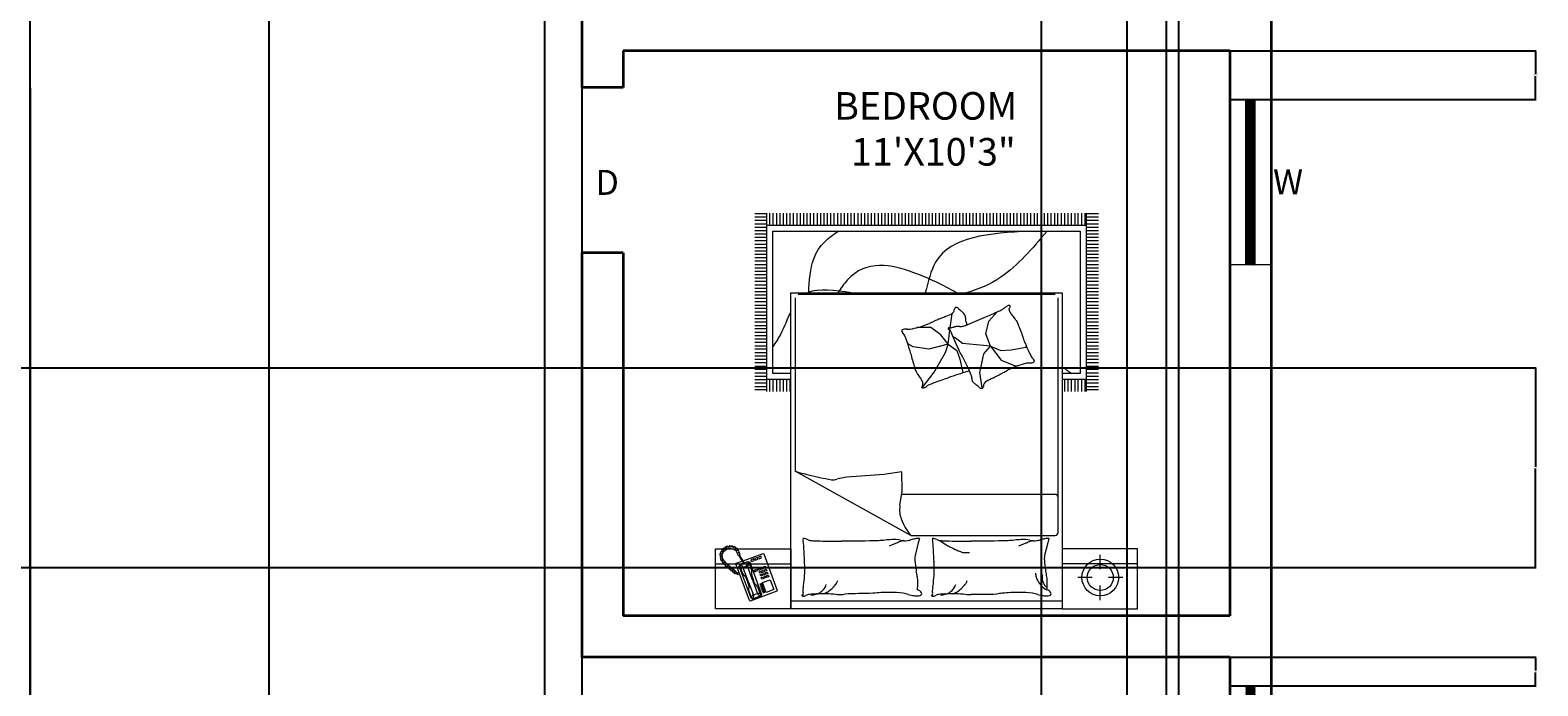
# Model space of a CAD drawing. Units: inches. Extents: x 318 to 927, y -1130 to 13.
# Tile 12 of 17: x 599 to 927, y -440 to -297. Entities that reach past the tile are written whole.
import ezdxf

# ---------------------------------------------------------------- set-up
doc = ezdxf.new("R2010")
doc.units = ezdxf.units.IN
doc.header["$MEASUREMENT"] = 0
for name, color, linetype, lineweight in [('A-ANNO-DIMS', 1, 'Continuous', 18), ('A-ANNO-IDEN', 1, 'Continuous', 13), ('A-AREA-IDEN', 8, 'Continuous', 18), ('A-GLAZ-PATT', 5, 'Continuous', 9), ('wall', 1, 'Continuous', 35), ('win', 5, 'Continuous', 18)]:
    doc.layers.add(name, color=color, linetype=linetype, lineweight=lineweight)
doc.layers.add('furniture', color=50, linetype='Continuous', lineweight=13, transparency=0.8)
doc.styles.add('DIM_FONT', font='SIMPLEX.shx', dxfattribs={"width": 0.8})
doc.styles.get("Standard").update_dxf_attribs({"font": 'arial.ttf'})
doc.dimstyles.get("Standard").update_dxf_attribs({"dimtxt": 0.18, "dimasz": 0.18, "dimexe": 0.18, "dimexo": 0.0625, "dimgap": 0.09, "dimtad": 0, "dimtih": 1, "dimtoh": 1, "dimdec": 1, "dimzin": 0, "dimdsep": 46, "dimlunit": 4, "dimtxsty": 'Standard', "dimcen": 0.09, "dimadec": 0, "dimazin": 0, "dimtfac": 1, "dimtdec": 1, "dimtofl": 0, "dimtmove": 0, "dimatfit": 3, "dimfxl": 1, "dimtolj": 1, "dimtzin": 0, "dimarcsym": 0})

# ---------------------------------------------------------------- blocks, each defined once
blk = doc.blocks.new('A$C4F634EDD')
for p, q in [((0, 2.629), (0, 2.229)), ((0.5, 2.629), (0, 2.629)), ((0.5, 2.629), (2.3, 2.629)), ((0.5, 0.529), (0.5, 2.629)), ((0.5, 2.229), (0.5, 2.629)), ((2.3, 2.629), (2.3, 0.529)), ((2.3, 2.629), (2.8, 2.629)), ((2.3, 2.229), (2.3, 2.629)), ((2.8, 2.629), (2.8, 2.229)), ((0.246, 2.57), (0.246, 2.473)), ((0.5, 2.577), (2.3, 2.577)), ((2.39, 2.507), (2.392, 2.511)), ((2.48, 2.262), (2.39, 2.507)), ((2.392, 2.511), (2.569, 2.577)), ((2.412, 2.501), (2.463, 2.52)), ((2.463, 2.52), (2.487, 2.454)), ((2.484, 2.523), (2.47, 2.518)), ((2.47, 2.518), (2.472, 2.513)), ((2.472, 2.513), (2.486, 2.518)), ((2.488, 2.513), (2.474, 2.507)), ((2.474, 2.507), (2.476, 2.502)), ((2.476, 2.502), (2.49, 2.507)), ((2.492, 2.502), (2.478, 2.497)), ((2.486, 2.518), (2.484, 2.523)), ((2.49, 2.507), (2.488, 2.513)), ((2.494, 2.497), (2.492, 2.502)), ((2.495, 2.533), (2.498, 2.545)), ((2.573, 2.319), (2.495, 2.533)), ((2.498, 2.545), (2.552, 2.564)), ((2.506, 2.545), (2.5, 2.539)), ((2.5, 2.539), (2.501, 2.531)), ((2.501, 2.531), (2.519, 2.484)), ((2.501, 2.531), (2.523, 2.521)), ((2.506, 2.545), (2.549, 2.561)), ((2.524, 2.526), (2.506, 2.545)), ((2.523, 2.521), (2.524, 2.526)), ((2.552, 2.442), (2.523, 2.521)), ((2.548, 2.535), (2.524, 2.526)), ((2.548, 2.535), (2.549, 2.561)), ((2.551, 2.532), (2.548, 2.535)), ((2.549, 2.561), (2.557, 2.56)), ((2.562, 2.554), (2.551, 2.532)), ((2.581, 2.452), (2.551, 2.532)), ((2.552, 2.564), (2.564, 2.558)), ((2.557, 2.56), (2.562, 2.554)), ((2.562, 2.554), (2.579, 2.506)), ((2.564, 2.558), (2.642, 2.346)), ((2.569, 2.577), (2.574, 2.574)), ((2.574, 2.574), (2.664, 2.33)), ((2.579, 2.506), (2.579, 2.496)), ((0.096, 2.42), (0.192, 2.42)), ((0.299, 2.42), (0.396, 2.42)), ((2.436, 2.435), (2.412, 2.501)), ((2.487, 2.454), (2.436, 2.435)), ((2.446, 2.415), (2.456, 2.418)), ((2.45, 2.404), (2.446, 2.415)), ((2.46, 2.408), (2.45, 2.404)), ((2.456, 2.418), (2.46, 2.408)), ((2.463, 2.421), (2.474, 2.425)), ((2.467, 2.41), (2.463, 2.421)), ((2.478, 2.414), (2.467, 2.41)), ((2.471, 2.402), (2.481, 2.405)), ((2.474, 2.425), (2.478, 2.414)), ((2.478, 2.497), (2.48, 2.491)), ((2.48, 2.491), (2.494, 2.497)), ((2.481, 2.428), (2.492, 2.431)), ((2.485, 2.417), (2.481, 2.428)), ((2.481, 2.405), (2.485, 2.395)), ((2.496, 2.491), (2.482, 2.486)), ((2.482, 2.486), (2.484, 2.481)), ((2.484, 2.481), (2.498, 2.486)), ((2.496, 2.421), (2.485, 2.417)), ((2.5, 2.481), (2.486, 2.475)), ((2.486, 2.475), (2.488, 2.47)), ((2.488, 2.47), (2.502, 2.475)), ((2.488, 2.408), (2.499, 2.412)), ((2.492, 2.397), (2.488, 2.408)), ((2.504, 2.47), (2.49, 2.465)), ((2.49, 2.465), (2.491, 2.46)), ((2.491, 2.46), (2.506, 2.465)), ((2.492, 2.431), (2.496, 2.421)), ((2.498, 2.486), (2.496, 2.491)), ((2.499, 2.412), (2.503, 2.401)), ((2.502, 2.475), (2.5, 2.481)), ((2.506, 2.465), (2.504, 2.47)), ((2.519, 2.484), (2.526, 2.476)), ((2.526, 2.476), (2.534, 2.469)), ((2.534, 2.469), (2.541, 2.457)), ((2.541, 2.457), (2.547, 2.44)), ((2.559, 2.406), (2.547, 2.44)), ((2.552, 2.442), (2.587, 2.346)), ((2.562, 2.393), (2.559, 2.406)), ((2.579, 2.496), (2.577, 2.485)), ((2.577, 2.485), (2.579, 2.472)), ((2.579, 2.472), (2.586, 2.454)), ((2.581, 2.452), (2.616, 2.356)), ((2.598, 2.42), (2.586, 2.454)), ((2.605, 2.409), (2.598, 2.42)), ((2.613, 2.402), (2.605, 2.409)), ((2.62, 2.394), (2.613, 2.402)), ((0, 2.33), (0.5, 2.33)), ((0.246, 2.366), (0.246, 2.27)), ((2.8, 2.33), (2.3, 2.33)), ((2.453, 2.395), (2.463, 2.399)), ((2.457, 2.384), (2.453, 2.395)), ((2.467, 2.388), (2.457, 2.384)), ((2.46, 2.376), (2.471, 2.379)), ((2.464, 2.365), (2.46, 2.376)), ((2.463, 2.399), (2.467, 2.388)), ((2.475, 2.369), (2.464, 2.365)), ((2.467, 2.356), (2.478, 2.36)), ((2.471, 2.345), (2.467, 2.356)), ((2.474, 2.391), (2.471, 2.402)), ((2.471, 2.379), (2.475, 2.369)), ((2.482, 2.349), (2.471, 2.345)), ((2.485, 2.395), (2.474, 2.391)), ((2.478, 2.382), (2.488, 2.386)), ((2.482, 2.371), (2.478, 2.382)), ((2.478, 2.36), (2.482, 2.349)), ((2.492, 2.375), (2.482, 2.371)), ((2.617, 2.309), (2.484, 2.26)), ((2.485, 2.363), (2.495, 2.367)), ((2.489, 2.352), (2.485, 2.363)), ((2.488, 2.386), (2.492, 2.375)), ((2.499, 2.356), (2.489, 2.352)), ((2.503, 2.401), (2.492, 2.397)), ((2.495, 2.389), (2.506, 2.392)), ((2.499, 2.378), (2.495, 2.389)), ((2.495, 2.367), (2.499, 2.356)), ((2.51, 2.382), (2.499, 2.378)), ((2.503, 2.369), (2.513, 2.373)), ((2.506, 2.358), (2.503, 2.369)), ((2.506, 2.392), (2.51, 2.382)), ((2.517, 2.362), (2.506, 2.358)), ((2.513, 2.373), (2.517, 2.362)), ((2.536, 2.305), (2.518, 2.299)), ((2.524, 2.377), (2.538, 2.382)), ((2.528, 2.366), (2.524, 2.377)), ((2.542, 2.371), (2.528, 2.366)), ((2.54, 2.294), (2.536, 2.305)), ((2.538, 2.382), (2.542, 2.371)), ((2.561, 2.314), (2.543, 2.308)), ((2.543, 2.308), (2.547, 2.297)), ((2.547, 2.297), (2.565, 2.304)), ((2.56, 2.382), (2.562, 2.393)), ((2.56, 2.372), (2.56, 2.382)), ((2.577, 2.324), (2.56, 2.372)), ((2.565, 2.304), (2.561, 2.314)), ((2.585, 2.313), (2.573, 2.319)), ((2.577, 2.324), (2.587, 2.346)), ((2.582, 2.318), (2.577, 2.324)), ((2.59, 2.317), (2.582, 2.318)), ((2.61, 2.322), (2.585, 2.313)), ((2.587, 2.346), (2.591, 2.343)), ((2.591, 2.343), (2.59, 2.317)), ((2.59, 2.317), (2.61, 2.324)), ((2.615, 2.352), (2.591, 2.343)), ((2.613, 2.331), (2.608, 2.329)), ((2.608, 2.329), (2.614, 2.314)), ((2.619, 2.317), (2.613, 2.331)), ((2.614, 2.314), (2.624, 2.298)), ((2.616, 2.356), (2.615, 2.352)), ((2.615, 2.352), (2.633, 2.332)), ((2.615, 2.326), (2.633, 2.332)), ((2.638, 2.346), (2.616, 2.356)), ((2.637, 2.332), (2.616, 2.324)), ((2.626, 2.307), (2.619, 2.317)), ((2.638, 2.346), (2.62, 2.394)), ((2.662, 2.325), (2.623, 2.311)), ((2.636, 2.292), (2.626, 2.307)), ((2.633, 2.332), (2.638, 2.339)), ((2.642, 2.346), (2.637, 2.332)), ((2.638, 2.339), (2.638, 2.346)), ((2.65, 2.398), (2.64, 2.395)), ((2.642, 2.39), (2.649, 2.391)), ((2.649, 2.391), (2.654, 2.39)), ((2.655, 2.397), (2.65, 2.398)), ((2.654, 2.39), (2.66, 2.388)), ((2.663, 2.392), (2.655, 2.397)), ((2.66, 2.388), (2.663, 2.387)), ((2.664, 2.33), (2.662, 2.325)), ((2.669, 2.394), (2.663, 2.392)), ((2.663, 2.387), (2.666, 2.388)), ((2.666, 2.388), (2.663, 2.383)), ((2.663, 2.383), (2.674, 2.374)), ((2.674, 2.394), (2.669, 2.394)), ((2.676, 2.391), (2.674, 2.394)), ((2.674, 2.38), (2.676, 2.391)), ((2.682, 2.386), (2.674, 2.38)), ((2.674, 2.374), (2.692, 2.359)), ((2.687, 2.381), (2.682, 2.386)), ((2.685, 2.369), (2.687, 2.381)), ((2.695, 2.376), (2.685, 2.369)), ((2.692, 2.359), (2.705, 2.347)), ((2.7, 2.371), (2.695, 2.376)), ((2.695, 2.36), (2.7, 2.371)), ((2.703, 2.368), (2.695, 2.36)), ((2.71, 2.362), (2.703, 2.368)), ((2.705, 2.347), (2.708, 2.348)), ((2.706, 2.351), (2.71, 2.362)), ((2.715, 2.358), (2.706, 2.351)), ((2.708, 2.348), (2.708, 2.344)), ((2.708, 2.344), (2.727, 2.328)), ((2.721, 2.352), (2.715, 2.358)), ((2.72, 2.34), (2.721, 2.352)), ((2.729, 2.347), (2.72, 2.34)), ((2.727, 2.328), (2.751, 2.298)), ((2.735, 2.342), (2.729, 2.347)), ((2.732, 2.33), (2.735, 2.342)), ((2.742, 2.335), (2.732, 2.33)), ((2.741, 2.317), (2.75, 2.325)), ((2.752, 2.322), (2.741, 2.317)), ((2.75, 2.325), (2.742, 2.335)), ((2.757, 2.314), (2.752, 2.322)), ((2.753, 2.304), (2.757, 2.314)), ((2.762, 2.308), (2.753, 2.304)), ((2.767, 2.3), (2.762, 2.308)), ((0, 2.229), (0.5, 2.229)), ((0.595, 2.191), (0.616, 2.274)), ((1.455, 2.191), (1.475, 2.274)), ((2.8, 2.229), (2.3, 2.229)), ((2.484, 2.26), (2.48, 2.262)), ((2.511, 2.296), (2.494, 2.289)), ((2.494, 2.289), (2.498, 2.279)), ((2.498, 2.279), (2.515, 2.285)), ((2.515, 2.285), (2.511, 2.296)), ((2.518, 2.299), (2.522, 2.288)), ((2.522, 2.288), (2.54, 2.294)), ((2.624, 2.298), (2.635, 2.282)), ((2.635, 2.282), (2.638, 2.273)), ((2.641, 2.283), (2.636, 2.292)), ((2.64, 2.271), (2.637, 2.266)), ((2.637, 2.266), (2.64, 2.257)), ((2.638, 2.273), (2.64, 2.271)), ((2.64, 2.257), (2.651, 2.259)), ((2.644, 2.274), (2.641, 2.283)), ((2.651, 2.259), (2.643, 2.249)), ((2.643, 2.249), (2.647, 2.24)), ((2.652, 2.272), (2.644, 2.274)), ((2.647, 2.24), (2.659, 2.243)), ((2.654, 2.263), (2.652, 2.272)), ((2.659, 2.243), (2.652, 2.231)), ((2.652, 2.231), (2.66, 2.225)), ((2.664, 2.241), (2.654, 2.263)), ((2.66, 2.225), (2.67, 2.231)), ((2.684, 2.229), (2.664, 2.241)), ((2.67, 2.231), (2.668, 2.219)), ((2.668, 2.219), (2.676, 2.215)), ((2.676, 2.215), (2.682, 2.224)), ((2.682, 2.224), (2.684, 2.213)), ((2.706, 2.226), (2.684, 2.229)), ((2.684, 2.213), (2.693, 2.212)), ((2.693, 2.212), (2.699, 2.222)), ((2.699, 2.222), (2.702, 2.21)), ((2.702, 2.21), (2.71, 2.21)), ((2.728, 2.232), (2.706, 2.226)), ((2.71, 2.21), (2.711, 2.222)), ((2.711, 2.222), (2.719, 2.214)), ((2.719, 2.214), (2.726, 2.215)), ((2.726, 2.215), (2.724, 2.227)), ((2.724, 2.227), (2.732, 2.216)), ((2.746, 2.248), (2.728, 2.232)), ((2.732, 2.216), (2.739, 2.221)), ((2.739, 2.221), (2.735, 2.231)), ((2.735, 2.231), (2.746, 2.226)), ((2.756, 2.27), (2.746, 2.248)), ((2.751, 2.231), (2.746, 2.242)), ((2.746, 2.242), (2.757, 2.235)), ((2.746, 2.226), (2.751, 2.231)), ((2.751, 2.298), (2.756, 2.27)), ((2.753, 2.25), (2.764, 2.25)), ((2.761, 2.242), (2.753, 2.25)), ((2.757, 2.292), (2.767, 2.3)), ((2.769, 2.29), (2.757, 2.292)), ((2.757, 2.235), (2.761, 2.242)), ((2.759, 2.279), (2.77, 2.283)), ((2.771, 2.273), (2.759, 2.279)), ((2.759, 2.264), (2.771, 2.264)), ((2.768, 2.256), (2.759, 2.264)), ((2.764, 2.25), (2.768, 2.256)), ((2.77, 2.283), (2.769, 2.29)), ((2.771, 2.264), (2.771, 2.273)), ((0.526, 2.121), (0.526, 0.562)), ((1.503, 2.141), (0.546, 2.141)), ((0.588, 2.161), (0.595, 2.191)), ((1.447, 2.161), (1.455, 2.191)), ((1.503, 2.141), (2.272, 1.714)), ((1.576, 1.943), (1.562, 1.848)), ((0.546, 1.868), (1.565, 1.868)), ((1.562, 1.848), (1.564, 1.718)), ((2.272, 0.562), (2.272, 1.714)), ((0.259, 1.175), (0.339, 1.175)), ((0.259, 1.153), (0.339, 1.153)), ((0.259, 1.13), (0.339, 1.13)), ((0.259, 1.108), (0.339, 1.108)), ((0.339, 0), (0.339, 1.185)), ((0.339, 1.105), (0.5, 1.105)), ((0.349, 1.105), (0.349, 1.185)), ((0.371, 1.105), (0.371, 1.185)), ((0.394, 1.105), (0.394, 1.185)), ((0.416, 1.105), (0.416, 1.185)), ((0.439, 1.105), (0.439, 1.185)), ((0.461, 1.105), (0.461, 1.185)), ((0.484, 1.105), (0.484, 1.185)), ((1.031, 1.161), (1.045, 1.058)), ((1.428, 1.161), (1.348, 1.057)), ((2.3, 1.105), (2.459, 1.105)), ((2.306, 1.105), (2.306, 1.185)), ((2.329, 1.105), (2.329, 1.185)), ((2.351, 1.105), (2.351, 1.185)), ((2.374, 1.105), (2.374, 1.185)), ((2.396, 1.105), (2.396, 1.185)), ((2.419, 1.105), (2.419, 1.185)), ((2.441, 1.105), (2.441, 1.185)), ((2.459, 1.185), (2.459, 0)), ((2.459, 1.175), (2.539, 1.175)), ((2.459, 1.153), (2.539, 1.153)), ((2.459, 1.13), (2.539, 1.13)), ((2.459, 1.108), (2.539, 1.108)), ((0.259, 1.085), (0.339, 1.085)), ((0.259, 1.063), (0.339, 1.063)), ((0.259, 1.04), (0.339, 1.04)), ((0.259, 1.018), (0.339, 1.018)), ((0.379, 1.065), (0.5, 1.065)), ((0.379, 0.12), (0.379, 1.065)), ((0.811, 1.015), (0.787, 1.012)), ((0.905, 0.977), (0.811, 1.015)), ((1.045, 1.058), (1.019, 0.936)), ((1.178, 0.97), (1.159, 1.059)), ((1.348, 1.057), (1.273, 0.927)), ((2.3, 1.065), (2.419, 1.065)), ((2.419, 1.065), (2.419, 0.12)), ((2.459, 1.085), (2.539, 1.085)), ((2.459, 1.063), (2.539, 1.063)), ((2.459, 1.04), (2.539, 1.04)), ((2.459, 1.018), (2.539, 1.018)), ((0.259, 0.995), (0.339, 0.995)), ((0.259, 0.973), (0.339, 0.973)), ((0.259, 0.95), (0.339, 0.95)), ((0.259, 0.928), (0.339, 0.928)), ((0.259, 0.905), (0.339, 0.905)), ((0.838, 0.909), (0.74, 0.891)), ((0.907, 0.912), (0.838, 0.909)), ((0.974, 0.884), (0.905, 0.977)), ((0.974, 0.884), (0.907, 0.912)), ((1.019, 0.936), (0.974, 0.884)), ((1.198, 0.913), (1.178, 0.97)), ((1.255, 0.871), (1.198, 0.913)), ((1.273, 0.927), (1.255, 0.871)), ((1.255, 0.871), (1.384, 0.903)), ((1.384, 0.903), (1.487, 0.889)), ((2.459, 0.995), (2.539, 0.995)), ((2.459, 0.973), (2.539, 0.973)), ((2.459, 0.95), (2.539, 0.95)), ((2.459, 0.928), (2.539, 0.928)), ((2.459, 0.905), (2.539, 0.905)), ((0.259, 0.883), (0.339, 0.883)), ((0.259, 0.86), (0.339, 0.86)), ((0.259, 0.838), (0.339, 0.838)), ((0.259, 0.815), (0.339, 0.815)), ((0.74, 0.891), (0.737, 0.885)), ((0.974, 0.884), (1.005, 0.802)), ((0.974, 0.884), (1.16, 0.866)), ((1.005, 0.802), (0.985, 0.719)), ((1.16, 0.866), (1.21, 0.829)), ((1.197, 0.885), (1.22, 0.829)), ((1.21, 0.829), (1.222, 0.821)), ((1.22, 0.829), (1.238, 0.786)), ((1.255, 0.871), (1.244, 0.777)), ((1.255, 0.871), (1.305, 0.808)), ((1.305, 0.808), (1.37, 0.761)), ((1.487, 0.889), (1.523, 0.869)), ((2.459, 0.883), (2.539, 0.883)), ((2.459, 0.86), (2.539, 0.86)), ((2.459, 0.838), (2.539, 0.838)), ((2.459, 0.815), (2.539, 0.815)), ((0.259, 0.793), (0.339, 0.793)), ((0.259, 0.77), (0.339, 0.77)), ((0.259, 0.748), (0.339, 0.748)), ((0.259, 0.725), (0.339, 0.725)), ((0.259, 0.703), (0.339, 0.703)), ((0.985, 0.719), (0.931, 0.657)), ((1.242, 0.763), (1.23, 0.668)), ((1.37, 0.761), (1.463, 0.761)), ((2.459, 0.793), (2.539, 0.793)), ((2.459, 0.77), (2.539, 0.77)), ((2.459, 0.748), (2.539, 0.748)), ((2.459, 0.725), (2.539, 0.725)), ((2.459, 0.703), (2.539, 0.703)), ((0.259, 0.68), (0.339, 0.68)), ((0.259, 0.658), (0.339, 0.658)), ((0.259, 0.635), (0.339, 0.635)), ((0.259, 0.613), (0.339, 0.613)), ((2.459, 0.68), (2.539, 0.68)), ((2.459, 0.658), (2.539, 0.658)), ((2.459, 0.635), (2.539, 0.635)), ((2.459, 0.613), (2.539, 0.613)), ((0.259, 0.59), (0.339, 0.59)), ((0.259, 0.568), (0.339, 0.568)), ((0.259, 0.545), (0.339, 0.545)), ((0.259, 0.523), (0.339, 0.523)), ((2.3, 0.529), (0.5, 0.529)), ((0.546, 0.542), (2.252, 0.542)), ((2.459, 0.59), (2.539, 0.59)), ((2.459, 0.568), (2.539, 0.568)), ((2.459, 0.545), (2.539, 0.545)), ((2.459, 0.523), (2.539, 0.523)), ((0.259, 0.5), (0.339, 0.5)), ((0.259, 0.478), (0.339, 0.478)), ((0.259, 0.455), (0.339, 0.455)), ((0.259, 0.433), (0.339, 0.433)), ((0.259, 0.41), (0.339, 0.41)), ((2.459, 0.5), (2.539, 0.5)), ((2.459, 0.478), (2.539, 0.478)), ((2.459, 0.455), (2.539, 0.455)), ((2.459, 0.433), (2.539, 0.433)), ((2.459, 0.41), (2.539, 0.41)), ((0.259, 0.388), (0.339, 0.388)), ((0.259, 0.365), (0.339, 0.365)), ((0.259, 0.343), (0.339, 0.343)), ((0.259, 0.32), (0.339, 0.32)), ((2.459, 0.388), (2.539, 0.388)), ((2.459, 0.365), (2.539, 0.365)), ((2.459, 0.343), (2.539, 0.343)), ((2.459, 0.32), (2.539, 0.32)), ((0.259, 0.298), (0.339, 0.298)), ((0.259, 0.275), (0.339, 0.275)), ((0.259, 0.253), (0.339, 0.253)), ((0.259, 0.23), (0.339, 0.23)), ((0.259, 0.208), (0.339, 0.208)), ((2.459, 0.298), (2.539, 0.298)), ((2.459, 0.275), (2.539, 0.275)), ((2.459, 0.253), (2.539, 0.253)), ((2.459, 0.23), (2.539, 0.23)), ((2.459, 0.208), (2.539, 0.208)), ((0.259, 0.185), (0.339, 0.185)), ((0.259, 0.163), (0.339, 0.163)), ((0.259, 0.14), (0.339, 0.14)), ((0.259, 0.118), (0.339, 0.118)), ((2.419, 0.12), (0.379, 0.12)), ((2.459, 0.185), (2.539, 0.185)), ((2.459, 0.163), (2.539, 0.163)), ((2.459, 0.14), (2.539, 0.14)), ((2.459, 0.118), (2.539, 0.118)), ((0.259, 0.095), (0.339, 0.095)), ((0.259, 0.073), (0.339, 0.073)), ((0.259, 0.05), (0.339, 0.05)), ((0.259, 0.028), (0.339, 0.028)), ((0.259, 0.005), (0.339, 0.005)), ((2.459, 0.08), (0.339, 0.08)), ((0.349, 0), (0.349, 0.08)), ((0.371, 0), (0.371, 0.08)), ((0.394, 0), (0.394, 0.08)), ((0.416, 0), (0.416, 0.08)), ((0.439, 0), (0.439, 0.08)), ((0.461, 0), (0.461, 0.08)), ((0.484, 0), (0.484, 0.08)), ((0.506, 0), (0.506, 0.08)), ((0.529, 0), (0.529, 0.08)), ((0.551, 0), (0.551, 0.08)), ((0.574, 0), (0.574, 0.08)), ((0.596, 0), (0.596, 0.08)), ((0.619, 0), (0.619, 0.08)), ((0.641, 0), (0.641, 0.08)), ((0.664, 0), (0.664, 0.08)), ((0.686, 0), (0.686, 0.08)), ((0.709, 0), (0.709, 0.08)), ((0.731, 0), (0.731, 0.08)), ((0.754, 0), (0.754, 0.08)), ((0.776, 0), (0.776, 0.08)), ((0.799, 0), (0.799, 0.08)), ((0.821, 0), (0.821, 0.08)), ((0.844, 0), (0.844, 0.08)), ((0.866, 0), (0.866, 0.08)), ((0.889, 0), (0.889, 0.08)), ((0.911, 0), (0.911, 0.08)), ((0.934, 0), (0.934, 0.08)), ((0.956, 0), (0.956, 0.08)), ((0.979, 0), (0.979, 0.08)), ((1.001, 0), (1.001, 0.08)), ((1.024, 0), (1.024, 0.08)), ((1.046, 0), (1.046, 0.08)), ((1.069, 0), (1.069, 0.08)), ((1.091, 0), (1.091, 0.08)), ((1.114, 0), (1.114, 0.08)), ((1.136, 0), (1.136, 0.08)), ((1.159, 0), (1.159, 0.08)), ((1.181, 0), (1.181, 0.08)), ((1.204, 0), (1.204, 0.08)), ((1.226, 0), (1.226, 0.08)), ((1.249, 0), (1.249, 0.08)), ((1.271, 0), (1.271, 0.08)), ((1.294, 0), (1.294, 0.08)), ((1.316, 0), (1.316, 0.08)), ((1.339, 0), (1.339, 0.08)), ((1.361, 0), (1.361, 0.08)), ((1.384, 0), (1.384, 0.08)), ((1.406, 0), (1.406, 0.08)), ((1.429, 0), (1.429, 0.08)), ((1.451, 0), (1.451, 0.08)), ((1.474, 0), (1.474, 0.08)), ((1.496, 0), (1.496, 0.08)), ((1.519, 0), (1.519, 0.08)), ((1.541, 0), (1.541, 0.08)), ((1.564, 0), (1.564, 0.08)), ((1.586, 0), (1.586, 0.08)), ((1.609, 0), (1.609, 0.08)), ((1.631, 0), (1.631, 0.08)), ((1.654, 0), (1.654, 0.08)), ((1.676, 0), (1.676, 0.08)), ((1.699, 0), (1.699, 0.08)), ((1.721, 0), (1.721, 0.08)), ((1.744, 0), (1.744, 0.08)), ((1.766, 0), (1.766, 0.08)), ((1.789, 0), (1.789, 0.08)), ((1.811, 0), (1.811, 0.08)), ((1.834, 0), (1.834, 0.08)), ((1.856, 0), (1.856, 0.08)), ((1.879, 0), (1.879, 0.08)), ((1.901, 0), (1.901, 0.08)), ((1.924, 0), (1.924, 0.08)), ((1.946, 0), (1.946, 0.08)), ((1.969, 0), (1.969, 0.08)), ((1.991, 0), (1.991, 0.08)), ((2.014, 0), (2.014, 0.08)), ((2.036, 0), (2.036, 0.08)), ((2.059, 0), (2.059, 0.08)), ((2.081, 0), (2.081, 0.08)), ((2.104, 0), (2.104, 0.08)), ((2.126, 0), (2.126, 0.08)), ((2.149, 0), (2.149, 0.08)), ((2.171, 0), (2.171, 0.08)), ((2.194, 0), (2.194, 0.08)), ((2.216, 0), (2.216, 0.08)), ((2.239, 0), (2.239, 0.08)), ((2.261, 0), (2.261, 0.08)), ((2.284, 0), (2.284, 0.08)), ((2.306, 0), (2.306, 0.08)), ((2.329, 0), (2.329, 0.08)), ((2.351, 0), (2.351, 0.08)), ((2.374, 0), (2.374, 0.08)), ((2.396, 0), (2.396, 0.08)), ((2.419, 0), (2.419, 0.08)), ((2.441, 0), (2.441, 0.08)), ((2.459, 0.095), (2.539, 0.095)), ((2.459, 0.073), (2.539, 0.073)), ((2.459, 0.05), (2.539, 0.05)), ((2.459, 0.028), (2.539, 0.028)), ((2.459, 0.005), (2.539, 0.005))]:
    blk.add_line(p, q)
for radius in [0.122, 0.0865]:
    blk.add_circle((0.246, 2.42), radius)
for centre, radius, start, end in [((0.585, 2.527), 0.0131, 101.2724, 206.5805), ((0.604, 2.537), 0.0342, 206.5805, 265.5998), ((0.6, 2.452), 0.0904, 90, 101.2724), ((1.09, 2.45), 0.492, 173.7676, 180), ((0.6, 2.381), 0.161, 81.5628, 90), ((0.537, 2.378), 0.14, 45.0976, 62.7964), ((0.579, 2.239), 0.305, 74.256, 81.5628), ((0.727, 2.765), 0.242, 254.256, 262.4531), ((0.785, 3.202), 0.683, 262.4531, 270), ((0.785, 3.568), 1.049, 270, 276.0867), ((0.84, 3.051), 0.529, 276.0867, 280.1899), ((1.16, -8.135), 10.667, 90.3015, 91.2158), ((1.117, 2.243), 0.29, 85.1982, 92.5386), ((1.214, 3.402), 0.873, 265.1982, 269.4243), ((1.432, 2.203), 0.392, 128.3886, 133.8115), ((1.236, 2.45), 0.0768, 117.2396, 128.3886), ((1.308, 2.31), 0.234, 110.8603, 117.2396), ((1.22, 4.023), 1.494, 269.4243, 271.9079), ((1.3, 2.436), 0.0992, 126.0864, 143.8234), ((1.3, 2.436), 0.0992, 105.9352, 126.0864), ((1.243, 3.35), 0.821, 271.9079, 275.2592), ((1.3, 2.436), 0.0992, 85.7841, 105.9352), ((1.313, 2.586), 0.0539, 275.2592, 300.6513), ((1.355, 2.515), 0.0289, 85.6975, 120.6513), ((1.356, 2.519), 0.0251, 68.2117, 85.6975), ((1.374, 2.529), 0.0156, 158.0096, 201.421), ((1.118, 2.541), 0.246, 347.8905, 351.8665), ((1.363, 2.533), 0.00428, 78.1069, 158.0096), ((1.329, 2.511), 0.0328, 351.8665, 21.421), ((1.365, 2.539), 0.00232, 258.1069, 19.564), ((1.364, 2.539), 0.00342, 19.564, 68.2117), ((1.444, 2.527), 0.0131, 101.2724, 206.5805), ((1.463, 2.537), 0.0342, 206.5805, 265.5998), ((1.459, 2.452), 0.0904, 90, 101.2724), ((1.949, 2.45), 0.492, 173.7676, 180), ((1.459, 2.381), 0.161, 81.5628, 90), ((1.438, 2.239), 0.305, 74.256, 81.5628), ((1.586, 2.765), 0.242, 254.256, 262.4531), ((1.644, 3.202), 0.683, 262.4531, 270), ((1.644, 3.568), 1.049, 270, 276.0867), ((1.479, 15.488), 12.966, 271.2243, 272.0532), ((1.97, 2.381), 0.152, 92.5386, 100.1899), ((1.976, 2.243), 0.29, 85.1982, 92.5386), ((2.073, 3.402), 0.873, 265.1982, 269.4243), ((2.291, 2.203), 0.392, 128.3886, 133.8115), ((2.095, 2.45), 0.0768, 117.2396, 128.3886), ((2.167, 2.31), 0.234, 110.8603, 117.2396), ((2.08, 4.023), 1.494, 269.4243, 271.9079), ((2.159, 2.436), 0.0992, 126.0864, 143.8234), ((2.159, 2.436), 0.0992, 105.9352, 126.0864), ((2.102, 3.35), 0.821, 271.9079, 275.2592), ((2.159, 2.436), 0.0992, 85.7841, 105.9352), ((2.172, 2.586), 0.0539, 275.2592, 300.6513), ((2.215, 2.515), 0.0289, 85.6975, 120.6513), ((2.215, 2.519), 0.0251, 68.2117, 85.6975), ((2.233, 2.529), 0.0156, 158.0096, 201.421), ((1.977, 2.541), 0.246, 347.8905, 351.8665), ((2.223, 2.533), 0.00428, 78.1069, 158.0096), ((2.188, 2.511), 0.0328, 351.8665, 21.421), ((2.224, 2.539), 0.00232, 258.1069, 19.564), ((2.223, 2.539), 0.00342, 19.564, 68.2117), ((0.802, 2.45), 0.204, 180, 189.6844), ((0.546, 2.414), 0.0899, 41.4429, 53.7359), ((1.47, 2.564), 0.882, 189.6844, 192.1984), ((0.574, 2.439), 0.0526, 25.3551, 41.4429), ((0.485, 2.397), 0.151, 21.8149, 25.3551), ((0.435, 2.376), 0.206, 18.7799, 21.8149), ((0.576, 2.425), 0.0562, 0, 18.7799), ((0.541, 2.425), 0.0915, 345.3149, 0), ((0.537, 2.378), 0.14, 27.3988, 45.0976), ((0.537, 2.378), 0.14, 16.515, 27.3988), ((0.537, 2.378), 0.14, 5.6311, 16.515), ((1.313, 2.363), 0.2, 151.6832, 156.9972), ((1.18, 2.434), 0.0493, 140.9651, 151.6832), ((1.317, 2.323), 0.225, 133.8115, 140.9651), ((1.3, 2.436), 0.0992, 143.8234, 161.5603), ((2.027, 2.366), 0.679, 176.6313, 181.6331), ((2.261, 2.353), 0.913, 172.3191, 176.6313), ((1.552, 2.448), 0.198, 167.8905, 172.3191), ((1.661, 2.45), 0.204, 180, 189.6844), ((2.33, 2.564), 0.882, 189.6844, 192.1984), ((2.172, 2.363), 0.2, 151.6832, 156.9972), ((2.039, 2.434), 0.0493, 140.9651, 151.6832), ((2.176, 2.323), 0.225, 133.8115, 140.9651), ((2.159, 2.436), 0.0992, 143.8234, 161.5603), ((2.886, 2.366), 0.679, 176.6313, 181.6331), ((3.12, 2.353), 0.913, 172.3191, 176.6313), ((2.411, 2.448), 0.198, 167.8905, 172.3191), ((0.298, 2.31), 0.317, 8.0051, 12.1984), ((-0.04, 2.263), 0.659, 2.6649, 8.0051), ((2.713, 2.386), 1.365, 181.6331, 183.055), ((14.966, 3.04), 13.636, 183.055, 183.5049), ((1.157, 2.31), 0.317, 8.0051, 12.1984), ((0.819, 2.263), 0.659, 2.6649, 8.0051), ((3.572, 2.386), 1.365, 181.6331, 183.055), ((15.825, 3.04), 13.636, 183.055, 183.5049), ((0.55, 2.29), 0.0677, 345.9548, 2.6649), ((0.473, 2.881), 0.739, 291.6577, 293.4844), ((0.473, 2.881), 0.739, 293.4844, 295.3111), ((1.13, 1.983), 0.272, 85.9172, 93.5552), ((1.146, 2.197), 0.058, 69.3257, 85.9172), ((0.987, 1.777), 0.507, 65.6735, 69.3257), ((0.606, 0.934), 1.432, 63.5015, 65.6735), ((1.105, 1.936), 0.313, 57.865, 63.5015), ((1.676, 2.226), 0.321, 183.5049, 189.9984), ((1.41, 2.29), 0.0677, 345.9548, 2.6649), ((1.332, 2.881), 0.739, 291.6577, 293.4844), ((1.332, 2.881), 0.739, 293.4844, 295.3111), ((2.535, 2.226), 0.321, 183.5049, 189.9984), ((0.546, 2.121), 0.02, 90, 180), ((0.589, 2.161), 0.000917, 165.9551, 274.0829), ((0.57, 2.43), 0.271, 274.0829, 279.4841), ((0.576, 2.39), 0.23, 279.4841, 287.3864), ((0.681, 2.056), 0.12, 96.4341, 107.3864), ((0.684, 2.03), 0.146, 78.4414, 96.4341), ((0.473, 2.881), 0.739, 287.1982, 289.428), ((0.759, 2.398), 0.23, 258.4414, 272.7491), ((0.473, 2.881), 0.739, 289.428, 291.6577), ((0.703, 3.572), 1.405, 272.7491, 274.6176), ((0.914, 0.959), 1.216, 92.6096, 94.6176), ((1.25, -19.84), 22.018, 90.3791, 91.0196), ((1.201, -3.54), 5.719, 89.7135, 90.9704), ((1.224, 1.014), 1.164, 86.426, 89.7135), ((0.884, 1.584), 0.729, 54.1737, 57.865), ((1.287, 2.03), 0.146, 77.131, 86.426), ((1.31, 2.128), 0.0453, 62.7159, 77.131), ((1.366, 2.237), 0.0767, 242.7159, 253.7788), ((1.369, 2.247), 0.0875, 253.7788, 262.8796), ((1.358, 2.162), 0.00132, 262.8796, 343.3022), ((1.341, 2.167), 0.0193, 343.3022, 9.9984), ((1.448, 2.161), 0.000917, 165.9551, 274.0829), ((1.429, 2.43), 0.271, 274.0829, 279.4841), ((1.436, 2.39), 0.23, 279.4841, 287.3864), ((1.215, 1.902), 0.375, 20.1488, 39.6445), ((1.54, 2.056), 0.12, 96.4341, 107.3864), ((1.543, 2.03), 0.146, 78.4414, 96.4341), ((1.332, 2.881), 0.739, 287.1982, 289.428), ((1.618, 2.398), 0.23, 258.4414, 272.7491), ((1.332, 2.881), 0.739, 289.428, 291.6577), ((1.562, 3.572), 1.405, 272.7491, 274.6176), ((1.773, 0.959), 1.216, 92.6096, 94.6176), ((2.109, -19.84), 22.018, 90.3791, 91.0196), ((2.06, -3.54), 5.719, 89.7135, 90.9704), ((2.083, 1.014), 1.164, 86.426, 89.7135), ((2.147, 2.03), 0.146, 77.131, 86.426), ((2.169, 2.128), 0.0453, 62.7159, 77.131), ((2.225, 2.237), 0.0767, 242.7159, 253.7788), ((2.228, 2.247), 0.0875, 253.7788, 262.8796), ((2.217, 2.162), 0.00132, 262.8796, 343.3022), ((2.2, 2.167), 0.0193, 343.3022, 9.9984), ((1.398, 1.969), 0.18, 351.8644, 20.1488), ((0.546, 1.888), 0.02, 180, 270), ((1.058, 5.464), 3.78, 277.692, 279.495), ((0.61, 18.053), 16.352, 273.757, 274.6239), ((1.419, 4.217), 2.516, 281.6741, 283.1904), ((2.038, 1.579), 0.194, 97.7304, 103.1904), ((2.019, 1.714), 0.0581, 79.2724, 97.7304), ((1.274, -2.223), 4.065, 77.0745, 79.2724), ((2.036, 1.098), 0.657, 74.0648, 77.0745), ((1.713, -0.034), 1.835, 72.2636, 74.0648), ((-0.417, 3.87), 3.097, 296.4147, 297.2902), ((0.986, 1.149), 0.0359, 297.2902, 3.2455), ((1.035, 1.152), 0.0127, 51.1864, 183.2455), ((0.999, 1.108), 0.0697, 45.8726, 51.1864), ((1.079, 1.19), 0.0452, 225.8726, 232.4713), ((1.285, 1.458), 0.383, 232.4713, 233.7837), ((0.668, 0.616), 0.66, 52.7849, 53.7837), ((0.936, 0.969), 0.218, 46.4776, 52.7849), ((1.033, 1.071), 0.0774, 35.8936, 46.4776), ((1.077, 1.103), 0.0226, 351.9508, 35.8936), ((-0.411, 5.908), 5.094, 289.0836, 290.1287), ((1.054, 1.911), 0.837, 290.1287, 292.7069), ((1.347, 1.212), 0.0792, 292.7069, 308.5854), ((1.434, 1.103), 0.0601, 110.3452, 128.5854), ((1.425, 1.126), 0.0352, 86.0516, 110.3452), ((1.5, 1.128), 0.0771, 169.5926, 177.2714), ((1.438, 1.131), 0.0153, 177.2714, 194.5709), ((1.461, 1.137), 0.0393, 194.5709, 206.8179), ((1.438, 1.14), 0.0142, 126.5792, 169.5926), ((1.74, 1.278), 0.352, 206.8179, 210.9056), ((1.427, 1.157), 0.00443, 13.2808, 86.0516), ((1.425, 1.156), 0.0063, 306.5792, 13.2808), ((0.642, 1.417), 0.43, 282.6252, 290.7486), ((0.574, 1.598), 0.624, 290.7486, 297.4921), ((-1.834, 6.224), 5.838, 297.4921, 297.8482), ((3.744, -4.334), 6.102, 117.4999, 117.8482), ((1.857, -0.71), 2.016, 116.4147, 117.4999), ((1.145, 1.093), 0.0458, 171.9508, 202.4162), ((2.032, 1.459), 1.005, 202.4162, 205.0529), ((1.092, 1.164), 0.117, 280.7366, 286.6085), ((2.649, 1.748), 1.687, 205.0529, 207.0884), ((0.227, 4.066), 3.145, 286.6085, 289.0836), ((1.605, 1.197), 0.194, 210.9056, 219.7005), ((1.393, 1.022), 0.081, 26.0735, 39.7005), ((1.289, 0.971), 0.197, 17.8396, 26.0735), ((-0.43, 0.417), 2.003, 15.2625, 17.8396), ((0.689, 0.983), 0.0058, 121.6917, 179.0386), ((0.7, 0.983), 0.0168, 179.0386, 229.4914), ((0.713, 0.945), 0.0509, 103.0402, 121.6917), ((0.64, 0.913), 0.0755, 26.3332, 49.4914), ((0.715, 0.936), 0.0599, 86.6119, 103.0402), ((-1.678, -0.234), 2.662, 25.1732, 26.3332), ((0.722, 1.059), 0.063, 266.6119, 282.6252), ((2.541, 1.692), 1.565, 207.0884, 209.936), ((0.999, 0.804), 0.214, 22.2355, 29.936), ((-0.088, 0.511), 1.648, 13.841, 15.2625), ((2.042, 1.036), 0.545, 193.841, 196.3122), ((0.569, 0.821), 0.18, 20.7081, 25.1732), ((0.227, 0.692), 0.545, 18.2369, 20.7081), ((2.31, 1.379), 1.648, 198.2369, 199.6584), ((2.644, 1.498), 2.003, 199.6584, 202.2355), ((1.691, 0.933), 0.18, 196.3122, 200.7773), ((4.012, 1.813), 2.662, 200.7773, 201.9373), ((1.612, 0.847), 0.0755, 201.9373, 225.0955), ((0.972, 0.814), 0.197, 202.2355, 210.4694), ((0.873, 0.756), 0.081, 210.4694, 224.0964), ((2.269, -2.19), 3.145, 111.0043, 113.4795), ((0.183, 0.409), 1.005, 18.0203, 19.3448), ((1.096, 0.706), 0.0458, 347.5549, 18.0203), ((1.183, 0.637), 0.117, 98.1216, 111.0043), ((1.176, 0.687), 0.0663, 85.4882, 98.1216), ((1.187, 0.824), 0.0712, 265.4882, 277.6784), ((1.173, 0.931), 0.179, 277.6784, 284.8807), ((1.269, 0.569), 0.195, 97.9822, 104.8807), ((1.259, 0.794), 0.0231, 202.2355, 252.8133), ((1.246, 0.729), 0.034, 85.7407, 97.9822), ((1.25, 0.772), 0.0092, 265.7407, 289.3799), ((1.251, 0.768), 0.00467, 289.3799, 72.8133), ((0.523, 2.558), 2.016, 292.0188, 293.104), ((-1.08, 6.316), 6.102, 293.104, 293.4523), ((3.672, -4.638), 5.838, 113.0962, 113.4523), ((1.627, 0.159), 0.624, 106.3527, 113.0962), ((1.572, 0.345), 0.43, 98.2293, 106.3527), ((1.52, 0.708), 0.063, 82.216, 98.2293), ((1.536, 0.83), 0.0599, 262.216, 278.6443), ((1.538, 0.821), 0.0509, 278.6443, 297.2959), ((1.547, 0.782), 0.0168, 354.6428, 45.0955), ((1.558, 0.781), 0.0058, 297.2959, 354.6428), ((0.675, 0.564), 0.194, 35.3015, 44.0964), ((0.546, 0.473), 0.352, 31.2138, 35.3015), ((0.851, 0.619), 0.0063, 130.9751, 197.6767), ((0.849, 0.618), 0.00443, 197.6767, 270.4475), ((0.837, 0.635), 0.0142, 310.9751, 353.9885), ((0.814, 0.635), 0.0393, 18.9668, 31.2138), ((0.849, 0.649), 0.0352, 270.4475, 294.7411), ((0.836, 0.643), 0.0153, 1.6673, 18.9668), ((0.775, 0.641), 0.0771, 353.9885, 1.6673), ((0.838, 0.672), 0.0601, 294.7411, 312.9813), ((0.933, 0.57), 0.0792, 117.1028, 132.9813), ((1.278, -0.105), 0.837, 114.5246, 117.1028), ((3.046, -3.978), 5.094, 113.4795, 114.5246), ((1.162, 0.691), 0.0226, 167.5549, 211.4977), ((1.209, 0.72), 0.0774, 211.4977, 222.0817), ((1.313, 0.814), 0.218, 222.0817, 228.389), ((1.607, 1.145), 0.66, 228.389, 229.3878), ((0.928, 0.353), 0.383, 48.0754, 49.3878), ((1.154, 0.604), 0.0452, 41.4767, 48.0754), ((1.24, 0.68), 0.0697, 221.4767, 226.7905), ((1.201, 0.639), 0.0127, 226.7905, 358.8496), ((1.249, 0.638), 0.0359, 112.8944, 178.8496), ((2.44, -2.182), 3.097, 112.0188, 112.8944)]:
    blk.add_arc(centre, radius, start, end)
for points in [[(0.439, 1.065), (0.46, 1.05), (0.48, 1.035), (0.5, 1.02)], [(1.9, 0.529), (2.006, 0.514), (2.113, 0.498), (2.189, 0.529)]]:
    blk.add_open_spline(points, degree=3)
for points, knots in [([(2.3, 0.653), (2.324, 0.703), (2.355, 0.791), (2.402, 0.861), (2.419, 0.887)], [1893.525221, 1893.525221, 1893.525221, 1893.525221, 2051.902476, 2146.74457, 2146.74457, 2146.74457, 2146.74457]), ([(0.599, 0.12), (0.696, 0.234), (0.852, 0.419), (1.054, 0.507), (1.136, 0.529)], [0, 0, 0, 0, 432.822832, 701.445452, 701.445452, 701.445452, 701.445452]), ([(0.719, 0.12), (0.979, 0.136), (1.326, 0.158), (1.387, 0.457), (1.408, 0.529)], [0, 0, 0, 0, 653.160442, 870.050857, 870.050857, 870.050857, 870.050857]), ([(1.202, 0.529), (1.289, 0.479), (1.514, 0.368), (1.826, 0.299), (1.968, 0.499), (1.987, 0.529)], [936.534237, 936.534237, 936.534237, 936.534237, 1243.285375, 1683.261222, 1758.254386, 1758.254386, 1758.254386, 1758.254386]), ([(2.18, 0.529), (2.18, 0.452), (2.155, 0.237), (2.049, 0.164), (1.985, 0.12)], [2202.034493, 2202.034493, 2202.034493, 2202.034493, 2357.807635, 2594.446174, 2594.446174, 2594.446174, 2594.446174])]:
    blk.add_open_spline(points, degree=3, knots=knots)
at = {"style": 'DIM_FONT', "width": 0.8, "flags": 9}
for tag, p in [('YSIZE', (0.5, 2.629)), ('XSIZE', (0.5, 2.629)), ('XSIZE', (2.298, 2.629)), ('YSIZE', (2.298, 2.629))]:
    blk.add_attdef(tag, p, '', height=0.0005, dxfattribs=at)
blk = doc.blocks.new('WIN-36IN')
for p, q in [((0, 36), (9, 36)), ((3.5, 36), (3.5, 0)), ((5.5, 36), (5.5, 0)), ((0, 0), (9, 0))]:
    blk.add_line(p, q)
blk = doc.blocks.new('*D27')
at = {"layer": 'A-ANNO-DIMS', "color": 0, "lineweight": -2, "transparency": 16777216}
for p, q in [((598.89, -309.98), (598.89, -1124.59)), ((718.89, -309.98), (718.89, -1124.59)), ((599.07, -1124.41), (658.5, -1124.41)), ((718.71, -1124.41), (659.28, -1124.41))]:
    blk.add_line(p, q, dxfattribs=at)
at = {"layer": 'A-ANNO-DIMS', "color": 0, "transparency": 16777216}
for points in [[(599.07, -1124.38), (599.07, -1124.44), (598.89, -1124.41)], [(718.71, -1124.38), (718.71, -1124.44), (718.89, -1124.41)]]:
    blk.add_solid(points, dxfattribs=at)
at = {"layer": 'Defpoints', "color": 0, "transparency": 16777216}
for p in [(598.89, -309.91), (718.89, -309.91), (718.89, -1124.41)]:
    blk.add_point(p, dxfattribs=at)
at = {"layer": 'A-ANNO-DIMS', "color": 0, "transparency": 16777216, "insert": (658.89, -1124.41), "char_height": 0.18, "attachment_point": 5}
blk.add_mtext('\\A1;10\'-0"', dxfattribs=at)
blk = doc.blocks.new('*D28')
at = {"layer": 'A-ANNO-DIMS', "color": 0, "lineweight": -2, "transparency": 16777216}
for p, q in [((650.89, -1033.85), (650.89, -25.23)), ((651.07, -25.41), (680.57, -25.41)), ((710.71, -25.41), (681.22, -25.41)), ((710.89, -1033.85), (710.89, -25.23))]:
    blk.add_line(p, q, dxfattribs=at)
at = {"layer": 'A-ANNO-DIMS', "color": 0, "transparency": 16777216}
for points in [[(651.07, -25.38), (651.07, -25.44), (650.89, -25.41)], [(710.71, -25.38), (710.71, -25.44), (710.89, -25.41)]]:
    blk.add_solid(points, dxfattribs=at)
at = {"layer": 'Defpoints', "color": 0, "transparency": 16777216}
for p in [(710.89, -25.41), (650.89, -1033.91), (710.89, -1033.91)]:
    blk.add_point(p, dxfattribs=at)
at = {"layer": 'A-ANNO-DIMS', "color": 0, "transparency": 16777216, "insert": (680.89, -25.41), "char_height": 0.18, "attachment_point": 5}
blk.add_mtext('\\A1;5\'-0"', dxfattribs=at)
blk = doc.blocks.new('*D29')
at = {"layer": 'A-ANNO-DIMS', "color": 0, "lineweight": -2, "transparency": 16777216}
for p, q in [((598.89, -1033.85), (598.89, -25.23)), ((599.07, -25.41), (624.56, -25.41)), ((650.71, -25.41), (625.23, -25.41)), ((650.89, -1033.85), (650.89, -25.23))]:
    blk.add_line(p, q, dxfattribs=at)
at = {"layer": 'A-ANNO-DIMS', "color": 0, "transparency": 16777216}
for points in [[(599.07, -25.38), (599.07, -25.44), (598.89, -25.41)], [(650.71, -25.38), (650.71, -25.44), (650.89, -25.41)]]:
    blk.add_solid(points, dxfattribs=at)
at = {"layer": 'Defpoints', "color": 0, "transparency": 16777216}
for p in [(650.89, -25.41), (598.89, -1033.91), (650.89, -1033.91)]:
    blk.add_point(p, dxfattribs=at)
at = {"layer": 'A-ANNO-DIMS', "color": 0, "transparency": 16777216, "insert": (624.89, -25.41), "char_height": 0.18, "attachment_point": 5}
blk.add_mtext('\\A1;4\'-4"', dxfattribs=at)
blk = doc.blocks.new('*D37')
at = {"layer": 'A-ANNO-DIMS', "color": 0, "lineweight": -2, "transparency": 16777216}
for p, q in [((531.96, -370.91), (926.57, -370.91)), ((926.39, -371.09), (926.39, -392.48)), ((926.39, -414.23), (926.39, -392.85)), ((531.96, -414.41), (926.57, -414.41))]:
    blk.add_line(p, q, dxfattribs=at)
at = {"layer": 'A-ANNO-DIMS', "color": 0, "transparency": 16777216}
for points in [[(926.36, -371.09), (926.42, -371.09), (926.39, -370.91)], [(926.36, -414.23), (926.42, -414.23), (926.39, -414.41)]]:
    blk.add_solid(points, dxfattribs=at)
at = {"layer": 'Defpoints', "color": 0, "transparency": 16777216}
for p in [(531.89, -370.91), (531.89, -414.41), (926.39, -414.41)]:
    blk.add_point(p, dxfattribs=at)
at = {"layer": 'A-ANNO-DIMS', "color": 0, "transparency": 16777216, "insert": (926.39, -392.66), "char_height": 0.18, "attachment_point": 5}
blk.add_mtext('\\A1;3\'-7 1/2"', dxfattribs=at)
blk = doc.blocks.new('*D43')
at = {"layer": 'A-ANNO-DIMS', "color": 0, "lineweight": -2, "transparency": 16777216}
for p, q in [((818.92, -537.33), (818.92, -25.23)), ((819.1, -25.41), (832.2, -25.41)), ((845.97, -25.41), (832.87, -25.41)), ((846.15, -539.79), (846.15, -25.23))]:
    blk.add_line(p, q, dxfattribs=at)
at = {"layer": 'A-ANNO-DIMS', "color": 0, "transparency": 16777216}
for points in [[(819.1, -25.38), (819.1, -25.44), (818.92, -25.41)], [(845.97, -25.38), (845.97, -25.44), (846.15, -25.41)]]:
    blk.add_solid(points, dxfattribs=at)
at = {"layer": 'Defpoints', "color": 0, "transparency": 16777216}
for p in [(846.15, -25.41), (818.92, -537.39), (846.15, -539.86)]:
    blk.add_point(p, dxfattribs=at)
at = {"layer": 'A-ANNO-DIMS', "color": 0, "transparency": 16777216, "insert": (832.53, -25.41), "char_height": 0.18, "attachment_point": 5}
blk.add_mtext('\\A1;2\'-3"', dxfattribs=at)
blk = doc.blocks.new('*D53')
at = {"layer": 'A-ANNO-DIMS', "color": 0, "lineweight": -2, "transparency": 16777216}
for p, q in [((837.57, -839.31), (837.57, -25.23)), ((837.75, -25.41), (842.6, -25.41)), ((848.66, -25.41), (843.82, -25.41)), ((848.84, -838.59), (848.84, -25.23))]:
    blk.add_line(p, q, dxfattribs=at)
at = {"layer": 'A-ANNO-DIMS', "color": 0, "transparency": 16777216}
for points in [[(837.75, -25.38), (837.75, -25.44), (837.57, -25.41)], [(848.66, -25.38), (848.66, -25.44), (848.84, -25.41)]]:
    blk.add_solid(points, dxfattribs=at)
at = {"layer": 'Defpoints', "color": 0, "transparency": 16777216}
for p in [(848.84, -25.41), (837.57, -839.37), (848.84, -838.66)]:
    blk.add_point(p, dxfattribs=at)
at = {"layer": 'A-ANNO-DIMS', "color": 0, "transparency": 16777216, "insert": (843.21, -25.41), "char_height": 0.18, "attachment_point": 5}
blk.add_mtext('\\A1;0\'-11 1/2"', dxfattribs=at)
blk = doc.blocks.new('*D61')
at = {"layer": 'A-ANNO-DIMS', "color": 0, "lineweight": -2, "transparency": 16777216}
for p, q in [((859.96, -301.91), (926.57, -301.91)), ((926.39, -302.09), (926.39, -307.03)), ((926.39, -312.34), (926.39, -307.4)), ((859.96, -312.52), (926.57, -312.52))]:
    blk.add_line(p, q, dxfattribs=at)
at = {"layer": 'A-ANNO-DIMS', "color": 0, "transparency": 16777216}
for points in [[(926.36, -302.09), (926.42, -302.09), (926.39, -301.91)], [(926.36, -312.34), (926.42, -312.34), (926.39, -312.52)]]:
    blk.add_solid(points, dxfattribs=at)
at = {"layer": 'Defpoints', "color": 0, "transparency": 16777216}
for p in [(859.89, -301.91), (859.89, -312.52), (926.39, -312.52)]:
    blk.add_point(p, dxfattribs=at)
at = {"layer": 'A-ANNO-DIMS', "color": 0, "transparency": 16777216, "insert": (926.39, -307.22), "char_height": 0.18, "attachment_point": 5}
blk.add_mtext('\\A1;0\'-10 1/2"', dxfattribs=at)
blk = doc.blocks.new('*D62')
at = {"layer": 'A-ANNO-DIMS', "color": 0, "lineweight": -2, "transparency": 16777216}
for p, q in [((859.96, -433.91), (926.57, -433.91)), ((926.39, -434.09), (926.39, -436.85)), ((926.39, -439.98), (926.39, -437.22)), ((859.96, -440.16), (926.57, -440.16))]:
    blk.add_line(p, q, dxfattribs=at)
at = {"layer": 'A-ANNO-DIMS', "color": 0, "transparency": 16777216}
for points in [[(926.36, -434.09), (926.42, -434.09), (926.39, -433.91)], [(926.36, -439.98), (926.42, -439.98), (926.39, -440.16)]]:
    blk.add_solid(points, dxfattribs=at)
at = {"layer": 'Defpoints', "color": 0, "transparency": 16777216}
for p in [(859.89, -433.91), (859.89, -440.16), (926.39, -440.16)]:
    blk.add_point(p, dxfattribs=at)
at = {"layer": 'A-ANNO-DIMS', "color": 0, "transparency": 16777216, "insert": (926.39, -437.04), "char_height": 0.18, "attachment_point": 5}
blk.add_mtext('\\A1;0\'-6"', dxfattribs=at)

msp = doc.modelspace()

# ---------------------------------------------------------------- hatches: boundary and pattern name
at = {"layer": 'A-GLAZ-PATT'}
h = msp.add_hatch(dxfattribs=at)
h.set_pattern_fill('ANSI31', color=256)
h.paths.add_polyline_path([(865.39, -312.52), (863.39, -312.52), (863.39, -348.52), (865.39, -348.52)])
h.paths.add_polyline_path([(865.39, -440.16), (863.39, -440.16), (863.39, -488.16), (865.39, -488.16)])
h.paths.add_polyline_path([(865.39, -635.51), (863.39, -635.51), (863.39, -683.51), (865.39, -683.51)])
h.paths.add_polyline_path([(865.39, -778.6), (863.39, -778.6), (863.39, -814.6), (865.39, -814.6)])
h.paths.add_polyline_path([(865.39, -834.21), (863.39, -834.21), (863.39, -870.21), (865.39, -870.21)])

# ---------------------------------------------------------------- linework, layer by layer
at = {"layer": 'wall'}
for p, q in [((868.89, -82.91), (868.89, -1042.91)), ((718.89, -135.91), (718.89, -309.91)), ((859.89, -301.91), (727.89, -301.91)), ((727.89, -301.91), (727.89, -309.91)), ((859.89, -301.91), (859.89, -424.91)), ((727.89, -309.91), (718.89, -309.91)), ((727.89, -345.91), (718.89, -345.91)), ((718.89, -345.91), (718.89, -433.91)), ((727.89, -345.91), (727.89, -424.91)), ((859.89, -424.91), (727.89, -424.91)), ((859.89, -433.91), (718.89, -433.91)), ((859.89, -433.91), (859.89, -691.91))]:
    msp.add_line(p, q, dxfattribs=at)

# ---------------------------------------------------------------- block references
at = {"layer": 'furniture', "xscale": 32.78135669785699, "yscale": 32.78135669785699, "zscale": 32.78135669785699, "rotation": 180}
msp.add_blockref('A$C4F634EDD', (839.79, -337.23), dxfattribs=at)
at = {"layer": 'win', "rotation": 180}
msp.add_blockref('WIN-36IN', (868.89, -312.52), dxfattribs=at)

# ---------------------------------------------------------------- texts
at = {"layer": 'A-ANNO-IDEN'}
for s, p in [('D', (721.89, -333.28)), ('W', (869.32, -333.18))]:
    msp.add_text(s, height=5.44, dxfattribs=at).set_placement(p)
at = {"layer": 'A-AREA-IDEN', "insert": (773.83, -310.9), "char_height": 6, "attachment_point": 1}
msp.add_mtext_dynamic_manual_height_columns('BEDROOM\\P  11\'X10\'3"', width=45.6749, gutter_width=1, heights=[0], dxfattribs=at)

# ---------------------------------------------------------------- dimensions: what is measured, and where the dimension line sits
at = {"layer": 'A-ANNO-DIMS'}
for base, p1, p2, picture, middle in [((650.89, -25.41), (598.89, -1033.91), (650.89, -1033.91), '*D29', (624.89, -25.41)), ((710.89, -25.41), (650.89, -1033.91), (710.89, -1033.91), '*D28', (680.89, -25.41)), ((846.15, -25.41), (818.92, -537.39), (846.15, -539.86), '*D43', (832.53, -25.41)), ((848.84, -25.41), (837.57, -839.37), (848.84, -838.66), '*D53', (843.21, -25.41)), ((718.89, -1124.41), (598.89, -309.91), (718.89, -309.91), '*D27', (658.89, -1124.41))]:
    dim = msp.add_linear_dim(base=base, p1=p1, p2=p2, dimstyle='Standard', override={"dimdec": 1, "dimlfac": 1, "dimrnd": 0, "dimzin": 1, "dimdsep": 46, "dimlunit": 4, "dimfrac": 2}, dxfattribs=at)
    dim.commit()
    dim.dimension.update_dxf_attribs({"geometry": picture, "text_midpoint": middle})
for base, p1, p2, picture, middle in [((926.39, -312.52), (859.89, -301.91), (859.89, -312.52), '*D61', (926.39, -307.22)), ((926.39, -414.41), (531.89, -370.91), (531.89, -414.41), '*D37', (926.39, -392.66)), ((926.3942, -440.1583), (859.8942, -433.9129), (859.8942, -440.1582), '*D62', (926.3942, -437.0356))]:
    dim = msp.add_linear_dim(base=base, p1=p1, p2=p2, angle=90, dimstyle='Standard', override={"dimdec": 1, "dimlfac": 1, "dimrnd": 0, "dimzin": 1, "dimdsep": 46, "dimlunit": 4, "dimfrac": 2}, dxfattribs=at)
    dim.commit()
    dim.dimension.update_dxf_attribs({"geometry": picture, "text_midpoint": middle})

doc.saveas('drawing.dxf')
